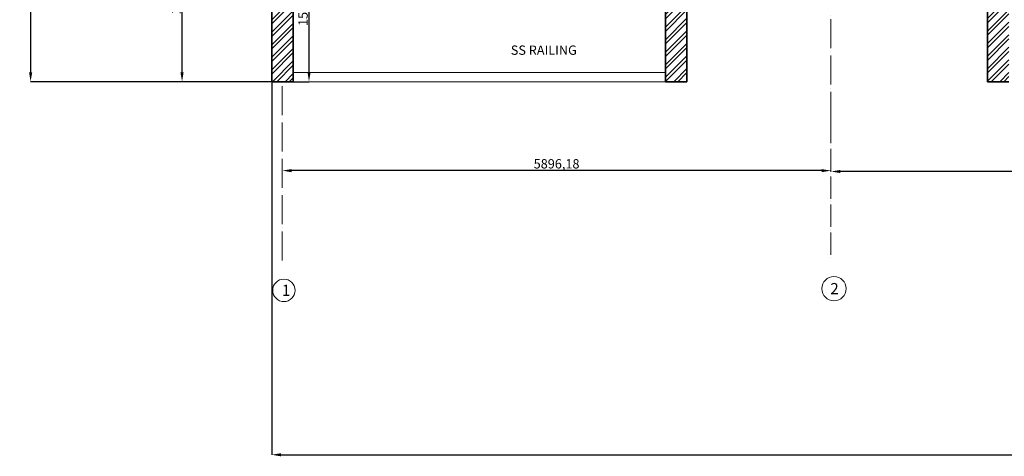
# Model space of a CAD drawing. Units: millimetres. Extents: x -3326 to 29338, y -16792 to 6002.
# Tile 1 of 21: x -3326 to 7252, y -16792 to -12098. Entities that reach past the tile are written whole.
import ezdxf

# ---------------------------------------------------------------- set-up
doc = ezdxf.new("R2010")
doc.units = ezdxf.units.MM
doc.header["$PDMODE"] = 35
doc.header["$PDSIZE"] = 5
doc.linetypes.add('ACAD_ISO04W100', pattern=[30, 24, -3, 0, -3])
for name, color, linetype, lineweight in [('A-ANNO-DIMS', 2, 'Continuous', 13), ('A-FLOR-RAIL', 8, 'Continuous', 20), ('A-GRID', 8, 'ACAD_ISO04W100', 13), ('A-GRID-IDEN', 7, 'Continuous', 18), ('A-WALL', 7, 'Continuous', 35), ('A-WALL-PATT', 252, 'Continuous', 13), ('txt', 7, 'Continuous', 18)]:
    doc.layers.add(name, color=color, linetype=linetype, lineweight=lineweight)
doc.styles.get("Standard").update_dxf_attribs({"font": 'arial.ttf'})
doc.dimstyles.new('ISO-25', dxfattribs={"dimtxt": 100, "dimasz": 100, "dimexe": 1.25, "dimexo": 0.625, "dimtad": 1, "dimtxsty": 'Standard', "dimcen": 2.5, "dimadec": 0, "dimazin": 0, "dimtfac": 1, "dimtmove": 0, "dimatfit": 3, "dimfxl": 1, "dimarcsym": 0})

# ---------------------------------------------------------------- blocks, each defined once
blk = doc.blocks.new('*D74')
at = {"layer": 'A-ANNO-DIMS', "color": 0, "lineweight": -2, "transparency": 16777216}
for p, q in [((-387, -11264), (-216, -11264)), ((-218, -12664), (-218, -11364)), ((-387, -12764), (-216, -12764))]:
    blk.add_line(p, q, dxfattribs=at)
at = {"layer": 'A-ANNO-DIMS', "color": 0, "transparency": 16777216}
for points in [[(-234, -11364), (-201, -11364), (-218, -11264)], [(-234, -12664), (-201, -12664), (-218, -12764)]]:
    blk.add_solid(points, dxfattribs=at)
at = {"layer": 'Defpoints', "color": 0, "transparency": 16777216}
for p in [(-388, -11264), (-218, -11264), (-388, -12764)]:
    blk.add_point(p, dxfattribs=at)
at = {"layer": 'A-ANNO-DIMS', "color": 0, "transparency": 16777216, "insert": (-269, -12014), "char_height": 100, "attachment_point": 5, "rotation": 90}
blk.add_mtext('1500', dxfattribs=at)
blk = doc.blocks.new('*D160')
at = {"layer": 'A-ANNO-DIMS', "color": 0, "lineweight": -2, "transparency": 16777216}
for p, q in [((5390, -13729), (5390, -13728)), ((11427, -13730), (5490, -13730)), ((11527, -13729), (11527, -13728))]:
    blk.add_line(p, q, dxfattribs=at)
at = {"layer": 'A-ANNO-DIMS', "color": 0, "transparency": 16777216}
for points in [[(5490, -13713), (5490, -13746), (5390, -13730)], [(11427, -13713), (11427, -13746), (11527, -13730)]]:
    blk.add_solid(points, dxfattribs=at)
at = {"layer": 'Defpoints', "color": 0, "transparency": 16777216}
for p in [(5390, -13730), (5390, -13730), (11527, -13730)]:
    blk.add_point(p, dxfattribs=at)
at = {"layer": 'A-ANNO-DIMS', "color": 0, "transparency": 16777216, "insert": (8459, -13669), "char_height": 100, "attachment_point": 5}
blk.add_mtext('6137,34', dxfattribs=at)
blk = doc.blocks.new('*D161')
at = {"layer": 'A-ANNO-DIMS', "color": 0, "lineweight": -2, "transparency": 16777216}
for p, q in [((-506, -13720), (-506, -13719)), ((5290, -13720), (-406, -13720)), ((5390, -13729), (5390, -13719))]:
    blk.add_line(p, q, dxfattribs=at)
at = {"layer": 'A-ANNO-DIMS', "color": 0, "transparency": 16777216}
for points in [[(-406, -13704), (-406, -13737), (-506, -13720)], [(5290, -13704), (5290, -13737), (5390, -13720)]]:
    blk.add_solid(points, dxfattribs=at)
at = {"layer": 'Defpoints', "color": 0, "transparency": 16777216}
for p in [(-506, -13720), (-506, -13720), (5390, -13730)]:
    blk.add_point(p, dxfattribs=at)
at = {"layer": 'A-ANNO-DIMS', "color": 0, "transparency": 16777216, "insert": (2442, -13660), "char_height": 100, "attachment_point": 5}
blk.add_mtext('5896,18', dxfattribs=at)
blk = doc.blocks.new('*D162')
at = {"layer": 'A-ANNO-DIMS', "color": 0, "lineweight": -2, "transparency": 16777216}
for p, q in [((-618, -11014), (-1583, -11014)), ((-1582, -12664), (-1582, -11114)), ((-618, -12764), (-1583, -12764))]:
    blk.add_line(p, q, dxfattribs=at)
at = {"layer": 'A-ANNO-DIMS', "color": 0, "transparency": 16777216}
for points in [[(-1599, -11114), (-1565, -11114), (-1582, -11014)], [(-1599, -12664), (-1565, -12664), (-1582, -12764)]]:
    blk.add_solid(points, dxfattribs=at)
at = {"layer": 'Defpoints', "color": 0, "transparency": 16777216}
for p in [(-1582, -11014), (-618, -11014), (-618, -12764)]:
    blk.add_point(p, dxfattribs=at)
at = {"layer": 'A-ANNO-DIMS', "color": 0, "transparency": 16777216, "insert": (-1634, -11889), "char_height": 100, "attachment_point": 5, "rotation": 90}
blk.add_mtext('1750', dxfattribs=at)
blk = doc.blocks.new('*D167')
at = {"layer": 'A-ANNO-DIMS', "color": 0, "lineweight": -2, "transparency": 16777216}
for p, q in [((-618, 3596), (-3210, 3596)), ((-3209, 3496), (-3209, -12664)), ((-618, -12764), (-3210, -12764))]:
    blk.add_line(p, q, dxfattribs=at)
at = {"layer": 'A-ANNO-DIMS', "color": 0, "transparency": 16777216}
for points in [[(-3226, 3496), (-3192, 3496), (-3209, 3596)], [(-3226, -12664), (-3192, -12664), (-3209, -12764)]]:
    blk.add_solid(points, dxfattribs=at)
at = {"layer": 'Defpoints', "color": 0, "transparency": 16777216}
for p in [(-618, 3596), (-3209, -12764), (-618, -12764)]:
    blk.add_point(p, dxfattribs=at)
at = {"layer": 'A-ANNO-DIMS', "color": 0, "transparency": 16777216, "insert": (-3261, -4584), "char_height": 100, "attachment_point": 5, "rotation": 90}
blk.add_mtext('16360', dxfattribs=at)
blk = doc.blocks.new('*D235')
at = {"layer": 'A-ANNO-DIMS', "color": 0, "lineweight": -2, "transparency": 16777216}
for p, q in [((-618, -12765), (-618, -16776)), ((29282, -12765), (29282, -16776)), ((-518, -16775), (29182, -16775))]:
    blk.add_line(p, q, dxfattribs=at)
at = {"layer": 'A-ANNO-DIMS', "color": 0, "transparency": 16777216}
for points in [[(-518, -16758), (-518, -16792), (-618, -16775)], [(29182, -16758), (29182, -16792), (29282, -16775)]]:
    blk.add_solid(points, dxfattribs=at)
at = {"layer": 'Defpoints', "color": 0, "transparency": 16777216}
for p in [(-618, -12764), (29282, -12764), (29282, -16775)]:
    blk.add_point(p, dxfattribs=at)
at = {"layer": 'A-ANNO-DIMS', "color": 0, "transparency": 16777216, "insert": (14332, -16723), "char_height": 100, "attachment_point": 5}
blk.add_mtext('29900', dxfattribs=at)

msp = doc.modelspace()

# ---------------------------------------------------------------- hatches: boundary and pattern name
at = {"layer": 'A-WALL-PATT'}
h = msp.add_hatch(dxfattribs=at)
h.set_pattern_fill('ANSI32', color=256, scale=10)
h.set_pattern_definition([(45, (-10476.65, 1e-12), (-67.35192, 67.35192), []), (45, (-10431.74, 1e-12), (-67.35192, 67.35192), [])])
h.paths.add_polyline_path([(7302.301, -11263.952), (7902.301, -11263.952), (7902.301, -11033.952), (7302.301, -11033.952), (7302.301, -8110.991), (7202.301, -8110.991), (7202.301, -11033.952), (6672.301, -11033.952), (6672.301, -11263.952), (7072.301, -11263.952), (7072.301, -12763.952), (7302.301, -12763.952)])
h.paths.add_polyline_path([(9152.301, -11033.952), (8802.301, -11033.952), (8802.301, -11044.19), (8802.545, -11044.19), (8802.545, -11124.19), (8802.301, -11263.952), (9152.301, -11263.952)])
h.paths.add_polyline_path([(3712.301, -8110.991), (3612.301, -8110.991), (3612.301, -11033.952), (3282.301, -11033.952), (3282.301, -11263.952), (3612.301, -11263.952), (3612.301, -12763.952), (3842.301, -12763.952), (3842.301, -11263.952), (4092.301, -11263.952), (4092.301, -11033.952), (3842.301, -11033.952), (3712.301, -11033.952)])
h.paths.add_polyline_path([(5172.301, -11033.952), (4692.301, -11033.952), (4692.301, -11263.952), (5172.301, -11263.952)])
h.paths.add_polyline_path([(6072.301, -11033.952), (5572.301, -11033.952), (5572.301, -11263.952), (6072.301, -11263.952)])
h.paths.add_polyline_path([(6072.301, -11263.952), (5972.301, -11263.952), (5972.301, -11663.952), (6072.301, -11663.952)])
h.paths.add_polyline_path([(4792.301, -11263.952), (4692.301, -11263.952), (4692.301, -11663.952), (4792.301, -11663.952)])
h.paths.add_polyline_path([(6402.301, -8110.991), (6272.301, -8110.991), (5572.301, -8110.991), (5572.301, -7200.401), (5342.301, -7200.401), (5342.301, -8110.991), (4642.301, -8110.991), (4512.301, -8110.991), (4512.301, -8210.991), (4642.301, -8210.991), (5342.301, -8210.991), (5342.301, -10513.952), (5572.301, -10513.952), (5572.301, -8210.991), (6272.301, -8210.991), (6402.301, -8210.991)])
h.paths.add_polyline_path([(232.301, -11033.952), (-217.699, -11033.952), (-217.699, -11263.952), (232.301, -11263.952)])
h.paths.add_polyline_path([(1482.301, -11033.952), (1132.301, -11033.952), (1132.301, -11044.8), (1132.987, -11044.8), (1132.987, -11124.8), (1132.301, -11263.952), (1482.301, -11263.952)])
h.paths.add_polyline_path([(-387.699, -11263.952), (-617.699, -11263.952), (-617.699, -12763.952), (-438.882, -12763.952), (-387.699, -12763.952)])
h.paths.add_polyline_path([(-387.699, -7150.401), (-215.519, -7150.401), (-215.519, -7050.401), (-617.699, -7050.401), (-617.699, -10763.952), (-387.699, -10763.952)])
h.paths.add_polyline_path([(1512.301, -5983.952), (1282.301, -5983.952), (1282.301, -6450.401), (-215.519, -6450.401), (-215.519, -6550.401), (4073.51, -6550.401), (4073.51, -6450.401), (1512.301, -6450.401)])
h.paths.add_polyline_path([(5773.51, -6450.401), (5573.51, -6450.401), (5573.51, -6550.401), (5773.51, -6550.401)])
h.paths.add_polyline_path([(5173.51, -6450.401), (4973.51, -6450.401), (4973.51, -6550.401), (5173.51, -6550.401)])
h.paths.add_polyline_path([(10982.301, -6450.401), (6673.51, -6450.401), (6673.51, -6550.401), (10982.301, -6550.401)])

# ---------------------------------------------------------------- linework, layer by layer
at = {"layer": 'A-FLOR-RAIL'}
for p, q in [((3612.301, -12663.952), (-387.699, -12663.952)), ((3612.301, -12763.952), (-387.699, -12763.952))]:
    msp.add_line(p, q, dxfattribs=at)
at = {"layer": 'A-GRID', "ltscale": 13}
for p, q in [((5389.966, -13184.889), (5389.966, -11255.956)), ((-506.217, -14684.889), (-506.217, -12755.956))]:
    msp.add_line(p, q, dxfattribs=at)
at = {"layer": 'A-GRID', "ltscale": 10}
msp.add_line((5389.966, -13184.889), (5389.966, -14674.996), dxfattribs=at)
at = {"layer": 'A-GRID-IDEN'}
for centre, radius in [((-487.268, -15007.214), 120.678), ((5422.042, -14988.866), 130.903)]:
    msp.add_circle(centre, radius, dxfattribs=at)
at = {"layer": 'A-WALL'}
for p, q in [((-617.699, -6450.401), (-617.699, -12763.952)), ((-387.699, -11263.952), (-387.699, -12763.952)), ((3612.301, -11263.952), (3612.301, -12763.952)), ((3842.301, -11263.952), (3842.301, -12763.952)), ((7072.301, -11263.952), (7072.301, -12763.952)), ((-438.882, -12763.952), (-617.699, -12763.952)), ((-387.699, -12763.952), (-438.882, -12763.952)), ((3842.301, -12763.952), (3612.301, -12763.952)), ((7302.301, -12763.952), (7072.301, -12763.952))]:
    msp.add_line(p, q, dxfattribs=at)

# ---------------------------------------------------------------- texts
at = {"layer": 'A-GRID-IDEN', "char_height": 120, "attachment_point": 1}
for s, insert in [('1', (-509.369, -14946.969)), ('2', (5382.301, -14928.62))]:
    msp.add_mtext_dynamic_manual_height_columns(s, width=463.74815, gutter_width=12.5, heights=[0], dxfattribs=dict(at, insert=insert))
at = {"layer": 'txt', "insert": (1949.93, -12375.166), "char_height": 100, "attachment_point": 1}
msp.add_mtext_dynamic_manual_height_columns('SS RAILING', width=1168.90663, gutter_width=12.5, heights=[0], dxfattribs=at)

# ---------------------------------------------------------------- dimensions: what is measured, and where the dimension line sits
at = {"layer": 'A-ANNO-DIMS'}
for base, p1, p2, picture, middle in [((-3209.046, -12763.952), (-617.699, 3596.048), (-617.699, -12763.952), '*D167', (-3260.762, -4583.952)), ((-1582.166, -11013.952), (-617.699, -12763.952), (-617.699, -11013.952), '*D162', (-1633.848, -11888.952)), ((-217.699, -11263.952), (-387.699, -12763.952), (-387.699, -11263.952), '*D74', (-269.382, -12013.952))]:
    dim = msp.add_linear_dim(base=base, p1=p1, p2=p2, angle=90, dimstyle='ISO-25', override={"dimclrd": 0, "dimclre": 0, "dimclrt": 0}, dxfattribs=at)
    dim.commit()
    dim.dimension.update_dxf_attribs({"geometry": picture, "text_midpoint": middle})
for base, p1, p2, override, picture, middle in [((29282.301, -16774.892), (-617.699, -12763.952), (29282.301, -12763.952), {"dimdec": 0, "dimlfac": 1, "dimrnd": 0, "dimzin": 0, "dimdsep": 46, "dimlunit": 2}, '*D235', (14332.301, -16723.21)), ((-506.217, -13720.422), (5389.966, -13729.669), (-506.217, -13720.422), {"dimclrd": 0, "dimclre": 0, "dimclrt": 0}, '*D161', (2441.874, -13659.702)), ((5389.9656, -13729.6686), (11527.3007, -13729.6686), (5389.9656, -13729.6686), {"dimclrd": 0, "dimclre": 0, "dimclrt": 0}, '*D160', (8458.6331, -13668.9481))]:
    dim = msp.add_linear_dim(base=base, p1=p1, p2=p2, dimstyle='ISO-25', override=override, dxfattribs=at)
    dim.commit()
    dim.dimension.update_dxf_attribs({"geometry": picture, "text_midpoint": middle})

doc.saveas('drawing.dxf')
